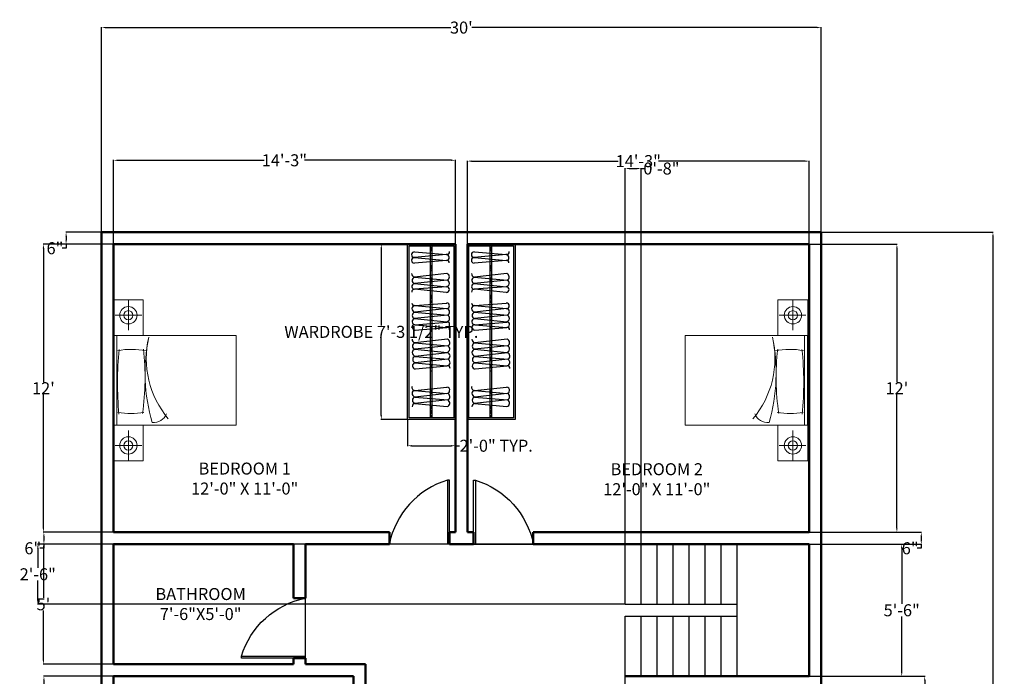
# Model space of a CAD drawing. Units: inches. Extents: x 20 to 32681, y 45 to 3082.
# Tile 3 of 5: x 20 to 512, y 344 to 672. Entities that reach past the tile are written whole.
import ezdxf

# ---------------------------------------------------------------- set-up
doc = ezdxf.new("R2010")
doc.units = ezdxf.units.IN
doc.header["$MEASUREMENT"] = 0
for name, color, linetype, lineweight in [('A-ANNO-DIMS', 2, 'Continuous', 18), ('A-AREA-IDEN', 7, 'Continuous', 25), ('A-DOOR', 4, 'Continuous', 25), ('A-FLOR-CASE', 32, 'Continuous', 25), ('A-FLOR-STRS', 3, 'Continuous', 25), ('A-FURN', 8, 'Continuous', 18), ('A-WALL', 7, 'Continuous', 50)]:
    doc.layers.add(name, color=color, linetype=linetype, lineweight=lineweight)
doc.styles.get("Standard").update_dxf_attribs({"font": 'arial.ttf'})
doc.dimstyles.get("Standard").update_dxf_attribs({"dimtxt": 6, "dimasz": 2, "dimexe": 0.18, "dimexo": 0.0625, "dimgap": 0.09, "dimtad": 0, "dimtih": 1, "dimtoh": 1, "dimdec": 0, "dimzin": 0, "dimdsep": 46, "dimlunit": 4, "dimtxsty": 'Standard', "dimcen": 0.09, "dimadec": 0, "dimazin": 0, "dimtfac": 1, "dimtdec": 0, "dimtofl": 0, "dimtmove": 0, "dimatfit": 3, "dimfxl": 1, "dimtolj": 1, "dimtzin": 0, "dimarcsym": 0})

# ---------------------------------------------------------------- blocks, each defined once
blk = doc.blocks.new('*D1')
at = {"layer": 'A-ANNO-DIMS', "color": 0, "lineweight": -2, "transparency": 16777216}
for p, q in [((60.79, 565.64), (60.79, 668.07)), ((62.79, 667.89), (235.61, 667.89)), ((418.79, 667.89), (245.97, 667.89)), ((420.79, 565.64), (420.79, 668.07))]:
    blk.add_line(p, q, dxfattribs=at)
at = {"layer": 'A-ANNO-DIMS', "color": 0, "transparency": 16777216}
for points in [[(62.79, 668.22), (62.79, 667.56), (60.79, 667.89)], [(418.79, 668.22), (418.79, 667.56), (420.79, 667.89)]]:
    blk.add_solid(points, dxfattribs=at)
at = {"layer": 'Defpoints', "color": 0, "transparency": 16777216}
for p in [(420.79, 667.89), (60.79, 565.58), (420.79, 565.58)]:
    blk.add_point(p, dxfattribs=at)
at = {"layer": 'A-ANNO-DIMS', "color": 0, "transparency": 16777216, "insert": (240.79, 667.89), "char_height": 6, "attachment_point": 5}
blk.add_mtext("\\A1;30'", dxfattribs=at)
blk = doc.blocks.new('DOOR')
for p, q in [((234.79, 441.58), (233.79, 441.58)), ((233.79, 441.58), (233.79, 409.58)), ((234.79, 409.58), (234.79, 441.58)), ((234.79, 409.58), (204.79, 409.58))]:
    blk.add_line(p, q)
blk.add_arc((245.82, 401.53), 41.82, 106.7253, 168.9058)
blk = doc.blocks.new('*D3')
at = {"layer": 'A-ANNO-DIMS', "color": 0, "lineweight": -2, "transparency": 16777216}
for p, q in [((414.85, 409.58), (461.22, 409.58)), ((461.04, 407.58), (461.04, 379.73)), ((461.04, 345.58), (461.04, 373.42)), ((414.85, 343.58), (461.22, 343.58))]:
    blk.add_line(p, q, dxfattribs=at)
at = {"layer": 'A-ANNO-DIMS', "color": 0, "transparency": 16777216}
for points in [[(460.7, 407.58), (461.37, 407.58), (461.04, 409.58)], [(460.7, 345.58), (461.37, 345.58), (461.04, 343.58)]]:
    blk.add_solid(points, dxfattribs=at)
at = {"layer": 'Defpoints', "color": 0, "transparency": 16777216}
for p in [(414.79, 409.58), (461.04, 409.58), (414.79, 343.58)]:
    blk.add_point(p, dxfattribs=at)
at = {"layer": 'A-ANNO-DIMS', "color": 0, "transparency": 16777216, "insert": (461.04, 376.58), "char_height": 6, "attachment_point": 5}
blk.add_mtext('\\A1;5\'-6"', dxfattribs=at)
blk = doc.blocks.new('CVBN')
for p, q in [((70.94, 1179.16), (70.94, 1191.01)), ((89.36, 1192.66), (89.36, 1168.36)), ((89.36, 1081.69), (89.36, 1192.39)), ((89.36, 1192.39), (89.36, 1168.09)), ((170.36, 1192.39), (89.36, 1192.39)), ((170.36, 1189.69), (89.36, 1189.69)), ((170.36, 1192.66), (170.36, 1168.36)), ((170.36, 1081.69), (170.36, 1192.39)), ((170.36, 1192.39), (170.36, 1168.09)), ((170.36, 1192.39), (170.36, 1168.09)), ((188.79, 1179.16), (188.79, 1191.01)), ((70.94, 1179.16), (56.8, 1179.16)), ((70.94, 1179.16), (84.43, 1179.16)), ((70.94, 1179.16), (70.94, 1166.85)), ((188.79, 1179.16), (175.29, 1179.16)), ((188.79, 1179.16), (202.93, 1179.16)), ((188.79, 1179.16), (188.79, 1166.85)), ((170.36, 1081.69), (89.36, 1081.69))]:
    blk.add_line(p, q)
for points in [[(56.96, 1192.66), (56.96, 1165.66), (89.36, 1165.66), (89.36, 1192.66)], [(202.76, 1192.66), (202.76, 1165.66), (170.36, 1165.66), (170.36, 1192.66)]]:
    blk.add_lwpolyline(points, close=True)
for centre, radius in [((70.94, 1179.16), 7.85), ((188.79, 1179.16), 7.85), ((70.94, 1179.16), 4.15), ((188.79, 1179.16), 4.15)]:
    blk.add_circle(centre, radius)
for centre, radius, start, end in [((127.34, 900.05), 288.94, 83.95302, 95.56263), ((165.23, 1177.16), 65.44, 169.91453, 190.68509), ((88.06, 1176.29), 69.84, 349.17608, 10.27064), ((136.55, 1004.48), 159.53, 78.24617, 106.34733), ((149.51, 1078.87), 84.09, 76.5636, 130.32358), ((132.8, 1394.24), 230.23, 261.76494, 276.28962), ((104.49, 1156.51), 12.88, 175.32687, 247.55878)]:
    blk.add_arc(centre, radius, start, end)
blk = doc.blocks.new('A$C1DC223CE')
for p, q in [((0, 600, -1029), (2200, 600, -1029)), ((0, 0, -1029), (0, 600, -1029)), ((20, 580, -1029), (2180, 580, -1029)), ((20, 20, -1029), (20, 580, -1029)), ((369, 495, -1029), (414, 88, -1029)), ((414, 85, -1029), (450, 501, -1029)), ((450, 499, -1029), (494, 87, -1029)), ((809, 498, -1029), (855, 91, -1029)), ((855, 88, -1029), (890, 504, -1029)), ((890, 502, -1029), (934, 89, -1029)), ((1194, 500, -1029), (1239, 93, -1029)), ((1239, 90, -1029), (1275, 506, -1029)), ((1275, 505, -1029), (1319, 92, -1029)), ((1319, 90, -1029), (1358, 496, -1029)), ((1363, 503, -1029), (1408, 96, -1029)), ((1408, 93, -1029), (1444, 509, -1029)), ((1444, 507, -1029), (1488, 95, -1029)), ((1488, 93, -1029), (1527, 499, -1029)), ((1565, 99, -1029), (1527, 499, -1029)), ((1874, 500, -1029), (1919, 93, -1029)), ((1919, 90, -1029), (1955, 506, -1029)), ((1955, 505, -1029), (1999, 92, -1029)), ((1999, 90, -1029), (2037, 496, -1029)), ((2180, 580, -1029), (2180, 20, -1029)), ((2200, 600, -1029), (2200, 0, -1029)), ((95, 88, -1029), (128, 488, -1029)), ((128, 486, -1029), (166, 85, -1029)), ((165, 88, -1029), (204, 488, -1029)), ((204, 488, -1029), (237, 85, -1029)), ((494, 85, -1029), (533, 491, -1029)), ((533, 488, -1029), (566, 85, -1029)), ((604, 488, -1029), (566, 88, -1029)), ((771, 91, -1029), (738, 491, -1029)), ((771, 91, -1029), (809, 491, -1029)), ((934, 88, -1029), (973, 494, -1029)), ((1011, 93, -1029), (979, 494, -1029)), ((1011, 93, -1029), (1045, 494, -1029)), ((1078, 93, -1029), (1045, 494, -1029)), ((1835, 92, -1029), (1795, 493, -1029)), ((1835, 93, -1029), (1874, 494, -1029)), ((2180, 309, -1029), (20, 309, -1029)), ((2180, 288, -1029), (20, 288, -1029)), ((45, 309, -1029), (45, 288, -1029)), ((50, 309, -1029), (50, 288, -1029)), ((63, 309, -1029), (63, 288, -1029)), ((77, 309, -1029), (77, 288, -1029)), ((83, 309, -1029), (83, 288, -1029)), ((273, 309, -1029), (273, 288, -1029)), ((278, 309, -1029), (278, 288, -1029)), ((291, 309, -1029), (291, 288, -1029)), ((304, 309, -1029), (304, 288, -1029)), ((313, 309, -1029), (313, 288, -1029)), ((333, 309, -1029), (333, 288, -1029)), ((428, 309, -1029), (428, 288, -1029)), ((433, 309, -1029), (433, 288, -1029)), ((446, 309, -1029), (446, 288, -1029)), ((459, 309, -1029), (459, 288, -1029)), ((468, 309, -1029), (468, 288, -1029)), ((488, 309, -1029), (488, 288, -1029)), ((645, 309, -1029), (645, 288, -1029)), ((650, 309, -1029), (650, 288, -1029)), ((660, 309, -1029), (660, 288, -1029)), ((678, 309, -1029), (678, 288, -1029)), ((683, 309, -1029), (683, 288, -1029)), ((687, 309, -1029), (687, 288, -1029)), ((716, 309, -1029), (716, 288, -1029)), ((725, 309, -1029), (725, 288, -1029)), ((731, 309, -1029), (731, 288, -1029)), ((877, 309, -1029), (877, 288, -1029)), ((888, 309, -1029), (888, 288, -1029)), ((952, 309, -1029), (952, 288, -1029)), ((959, 309, -1029), (959, 288, -1029)), ((1036, 309, -1029), (1036, 288, -1029)), ((1047, 309, -1029), (1047, 288, -1029)), ((1273, 309, -1029), (1273, 288, -1029)), ((1308, 309, -1029), (1308, 288, -1029)), ((1319, 309, -1029), (1319, 288, -1029)), ((1330, 309, -1029), (1330, 288, -1029)), ((1341, 309, -1029), (1341, 288, -1029)), ((1346, 309, -1029), (1346, 288, -1029)), ((1421, 309, -1029), (1421, 288, -1029)), ((1432, 309, -1029), (1432, 288, -1029)), ((1446, 309, -1029), (1446, 288, -1029)), ((1448, 309, -1029), (1448, 288, -1029)), ((1459, 309, -1029), (1459, 288, -1029)), ((1466, 309, -1029), (1466, 288, -1029)), ((1513, 309, -1029), (1513, 288, -1029)), ((1521, 309, -1029), (1521, 288, -1029)), ((1532, 309, -1029), (1532, 288, -1029)), ((1544, 309, -1029), (1544, 288, -1029)), ((1553, 309, -1029), (1553, 288, -1029)), ((1592, 309, -1029), (1592, 288, -1029)), ((1836, 309, -1029), (1836, 288, -1029)), ((1844, 309, -1029), (1844, 288, -1029)), ((1856, 309, -1029), (1856, 288, -1029)), ((1865, 309, -1029), (1865, 288, -1029)), ((1874, 309, -1029), (1874, 288, -1029)), ((2043, 309, -1029), (2043, 288, -1029)), ((2048, 309, -1029), (2048, 288, -1029)), ((2066, 309, -1029), (2066, 288, -1029)), ((2091, 309, -1029), (2091, 288, -1029)), ((2099, 309, -1029), (2099, 288, -1029)), ((2109, 309, -1029), (2109, 288, -1029)), ((2127, 309, -1029), (2127, 288, -1029)), ((2153, 309, -1029), (2153, 288, -1029)), ((2164, 309, -1029), (2164, 288, -1029)), ((2200, 0, -1029), (0, 0, -1029)), ((2180, 20, -1029), (20, 20, -1029))]:
    blk.add_line(p, q)
for centre, radius, start, end in [((98, 496, -1029), 31, 344.0746, 99.05), ((166, 484, -1029), 38.5, 94.0153, 178.1465), ((171, 491, -1029), 32.8, 355.4947, 103.6477), ((232, 494, -1029), 29, 86.5574, 190.9577), ((411, 482, -1029), 43.6, 25.0318, 162.7252), ((490, 482, -1029), 43.5, 11.8045, 156.7744), ((571, 487, -1029), 38.5, 94.0153, 178.1465), ((566, 487, -1029), 38.5, 1.8535, 85.9847), ((769, 494, -1029), 31.7, 82.3676, 185.3857), ((778, 494, -1029), 31.7, 354.6143, 97.6324), ((851, 485, -1029), 43.6, 25.0318, 162.7252), ((930, 485, -1029), 43.5, 11.8045, 156.7744), ((1002, 504, -1029), 25.4, 75.2713, 202.7917), ((1013, 497, -1029), 31.7, 354.6143, 97.6324), ((1068, 504, -1029), 25.4, 75.2713, 202.7917), ((1235, 488, -1029), 43.6, 25.0318, 162.7252), ((1315, 487, -1029), 43.5, 11.8045, 156.7744), ((1405, 490, -1029), 43.6, 25.0318, 162.7252), ((1484, 490, -1029), 43.5, 11.8045, 156.7744), ((1558, 502, -1029), 31.7, 82.3676, 185.3857), ((1830, 494, -1029), 35.9, 71.1886, 180.696), ((1842, 497, -1029), 31.7, 354.6143, 97.6324), ((1915, 488, -1029), 43.6, 25.0318, 162.7252), ((1995, 487, -1029), 43.5, 11.8045, 156.7744), ((133, 89, -1029), 38.5, 181.8535, 265.9847), ((135, 82, -1029), 31.7, 262.3676, 5.3857), ((204, 89, -1029), 38.5, 181.8535, 265.9847), ((205, 82, -1029), 31.7, 262.3676, 5.3857), ((364, 104, -1029), 52.8, 272.4772, 342.818), ((454, 98, -1029), 41.7, 197.7504, 344.2252), ((536, 96, -1029), 42.8, 195.0477, 270), ((529, 90, -1029), 37.5, 280.6806, 351.7243), ((597, 85, -1029), 31.7, 174.6143, 277.6324), ((742, 84, -1029), 30.1, 267.7337, 14.6117), ((809, 92, -1029), 38.5, 181.8535, 265.9847), ((804, 106, -1029), 52.8, 272.4772, 342.818), ((894, 101, -1029), 41.7, 197.7504, 344.2252), ((976, 99, -1029), 42.8, 195.0477, 270), ((973, 95, -1029), 38.5, 274.0153, 358.1465), ((1040, 86, -1029), 29.8, 166.1294, 272.546), ((1039, 95, -1029), 38.5, 274.0153, 358.1465), ((1189, 109, -1029), 52.8, 272.4772, 342.818), ((1279, 103, -1029), 41.7, 197.7504, 344.2252), ((1360, 101, -1029), 42.8, 195.0477, 270), ((1358, 111, -1029), 52.8, 272.4772, 342.818), ((1448, 106, -1029), 41.7, 197.7504, 344.2252), ((1530, 104, -1029), 42.8, 195.0477, 270), ((1527, 100, -1029), 38.5, 274.0153, 358.1465), ((1799, 90, -1029), 36.2, 250.2345, 4.119), ((1874, 94, -1029), 38.5, 181.8535, 265.9847), ((1869, 109, -1029), 52.8, 272.4772, 342.818), ((1959, 103, -1029), 41.7, 197.7504, 344.2252), ((2040, 101, -1029), 42.8, 195.0477, 270)]:
    blk.add_arc(centre, radius, start, end)
blk = doc.blocks.new('*D12')
at = {"layer": 'A-ANNO-DIMS', "color": 0, "lineweight": -2, "transparency": 16777216}
for p, q in [((60.73, 565.58), (42.93, 565.58)), ((43.11, 563.58), (43.11, 561.58)), ((43.11, 557.58), (41.11, 557.58)), ((60.73, 559.58), (42.93, 559.58)), ((43.11, 559.58), (43.11, 557.58))]:
    blk.add_line(p, q, dxfattribs=at)
at = {"layer": 'A-ANNO-DIMS', "color": 0, "transparency": 16777216}
for points in [[(42.78, 563.58), (43.44, 563.58), (43.11, 565.58)], [(42.78, 561.58), (43.44, 561.58), (43.11, 559.58)]]:
    blk.add_solid(points, dxfattribs=at)
at = {"layer": 'Defpoints', "color": 0, "transparency": 16777216}
for p in [(60.79, 565.58), (43.11, 559.58), (60.79, 559.58)]:
    blk.add_point(p, dxfattribs=at)
at = {"layer": 'A-ANNO-DIMS', "color": 0, "transparency": 16777216, "insert": (37.55, 557.58), "char_height": 6, "attachment_point": 5}
blk.add_mtext('\\A1;6"', dxfattribs=at)
blk = doc.blocks.new('*D13')
at = {"layer": 'A-ANNO-DIMS', "color": 0, "lineweight": -2, "transparency": 16777216}
for p, q in [((66.73, 559.58), (31.59, 559.58)), ((31.77, 557.58), (31.77, 490.68)), ((31.77, 417.58), (31.77, 484.47)), ((66.73, 415.58), (31.59, 415.58))]:
    blk.add_line(p, q, dxfattribs=at)
at = {"layer": 'A-ANNO-DIMS', "color": 0, "transparency": 16777216}
for points in [[(31.43, 557.58), (32.1, 557.58), (31.77, 559.58)], [(31.43, 417.58), (32.1, 417.58), (31.77, 415.58)]]:
    blk.add_solid(points, dxfattribs=at)
at = {"layer": 'Defpoints', "color": 0, "transparency": 16777216}
for p in [(66.79, 559.58), (31.77, 415.58), (66.79, 415.58)]:
    blk.add_point(p, dxfattribs=at)
at = {"layer": 'A-ANNO-DIMS', "color": 0, "transparency": 16777216, "insert": (31.77, 487.58), "char_height": 6, "attachment_point": 5}
blk.add_mtext("\\A1;12'", dxfattribs=at)
blk = doc.blocks.new('*D14')
at = {"layer": 'A-ANNO-DIMS', "color": 0, "lineweight": -2, "transparency": 16777216}
for p, q in [((66.73, 415.58), (31.83, 415.58)), ((66.73, 409.58), (31.83, 409.58)), ((32.01, 413.58), (32.01, 411.58)), ((32.01, 409.58), (32.01, 407.58)), ((32.01, 407.58), (30.01, 407.58))]:
    blk.add_line(p, q, dxfattribs=at)
at = {"layer": 'A-ANNO-DIMS', "color": 0, "transparency": 16777216}
for points in [[(31.68, 413.58), (32.34, 413.58), (32.01, 415.58)], [(31.68, 411.58), (32.34, 411.58), (32.01, 409.58)]]:
    blk.add_solid(points, dxfattribs=at)
at = {"layer": 'Defpoints', "color": 0, "transparency": 16777216}
for p in [(66.79, 415.58), (32.01, 409.58), (66.79, 409.58)]:
    blk.add_point(p, dxfattribs=at)
at = {"layer": 'A-ANNO-DIMS', "color": 0, "transparency": 16777216, "insert": (26.46, 407.58), "char_height": 6, "attachment_point": 5}
blk.add_mtext('\\A1;6"', dxfattribs=at)
blk = doc.blocks.new('*D15')
at = {"layer": 'A-ANNO-DIMS', "color": 0, "lineweight": -2, "transparency": 16777216}
for p, q in [((66.73, 409.58), (31.59, 409.58)), ((31.77, 407.58), (31.77, 382.72)), ((31.77, 351.58), (31.77, 376.43)), ((66.73, 349.58), (31.59, 349.58))]:
    blk.add_line(p, q, dxfattribs=at)
at = {"layer": 'A-ANNO-DIMS', "color": 0, "transparency": 16777216}
for points in [[(31.43, 407.58), (32.1, 407.58), (31.77, 409.58)], [(31.43, 351.58), (32.1, 351.58), (31.77, 349.58)]]:
    blk.add_solid(points, dxfattribs=at)
at = {"layer": 'Defpoints', "color": 0, "transparency": 16777216}
for p in [(66.79, 409.58), (31.77, 349.58), (66.79, 349.58)]:
    blk.add_point(p, dxfattribs=at)
at = {"layer": 'A-ANNO-DIMS', "color": 0, "transparency": 16777216, "insert": (31.77, 379.58), "char_height": 6, "attachment_point": 5}
blk.add_mtext("\\A1;5'", dxfattribs=at)
blk = doc.blocks.new('*D16')
at = {"layer": 'A-ANNO-DIMS', "color": 0, "lineweight": -2, "transparency": 16777216}
for p, q in [((66.73, 343.58), (31.84, 343.58)), ((32.02, 341.58), (32.02, 298.73)), ((32.02, 249.58), (32.02, 292.42)), ((66.73, 247.58), (31.84, 247.58))]:
    blk.add_line(p, q, dxfattribs=at)
at = {"layer": 'A-ANNO-DIMS', "color": 0, "transparency": 16777216}
for points in [[(31.69, 341.58), (32.35, 341.58), (32.02, 343.58)], [(31.69, 249.58), (32.35, 249.58), (32.02, 247.58)]]:
    blk.add_solid(points, dxfattribs=at)
at = {"layer": 'Defpoints', "color": 0, "transparency": 16777216}
for p in [(66.79, 343.58), (32.02, 247.58), (66.79, 247.58)]:
    blk.add_point(p, dxfattribs=at)
at = {"layer": 'A-ANNO-DIMS', "color": 0, "transparency": 16777216, "insert": (32.02, 295.58), "char_height": 6, "attachment_point": 5}
blk.add_mtext("\\A1;8'", dxfattribs=at)
blk = doc.blocks.new('*D22')
at = {"layer": 'A-ANNO-DIMS', "color": 0, "lineweight": -2, "transparency": 16777216}
for p, q in [((414.85, 343.58), (472.74, 343.58)), ((472.56, 341.58), (472.56, 339.58)), ((414.85, 337.58), (472.74, 337.58)), ((472.56, 335.58), (470.56, 335.58)), ((472.56, 337.58), (472.56, 335.58))]:
    blk.add_line(p, q, dxfattribs=at)
at = {"layer": 'A-ANNO-DIMS', "color": 0, "transparency": 16777216}
for points in [[(472.23, 341.58), (472.89, 341.58), (472.56, 343.58)], [(472.23, 339.58), (472.89, 339.58), (472.56, 337.58)]]:
    blk.add_solid(points, dxfattribs=at)
at = {"layer": 'Defpoints', "color": 0, "transparency": 16777216}
for p in [(414.79, 343.58), (414.79, 337.58), (472.56, 337.58)]:
    blk.add_point(p, dxfattribs=at)
at = {"layer": 'A-ANNO-DIMS', "color": 0, "transparency": 16777216, "insert": (467, 335.58), "char_height": 6, "attachment_point": 5}
blk.add_mtext('\\A1;6"', dxfattribs=at)
blk = doc.blocks.new('*D23')
at = {"layer": 'A-ANNO-DIMS', "color": 0, "lineweight": -2, "transparency": 16777216}
for p, q in [((414.85, 559.58), (458.81, 559.58)), ((458.63, 557.58), (458.63, 490.68)), ((458.63, 417.58), (458.63, 484.47)), ((414.85, 415.58), (458.81, 415.58))]:
    blk.add_line(p, q, dxfattribs=at)
at = {"layer": 'A-ANNO-DIMS', "color": 0, "transparency": 16777216}
for points in [[(458.3, 557.58), (458.97, 557.58), (458.63, 559.58)], [(458.3, 417.58), (458.97, 417.58), (458.63, 415.58)]]:
    blk.add_solid(points, dxfattribs=at)
at = {"layer": 'Defpoints', "color": 0, "transparency": 16777216}
for p in [(414.79, 559.58), (458.63, 559.58), (414.79, 415.58)]:
    blk.add_point(p, dxfattribs=at)
at = {"layer": 'A-ANNO-DIMS', "color": 0, "transparency": 16777216, "insert": (458.63, 487.58), "char_height": 6, "attachment_point": 5}
blk.add_mtext("\\A1;12'", dxfattribs=at)
blk = doc.blocks.new('*D24')
at = {"layer": 'A-ANNO-DIMS', "color": 0, "lineweight": -2, "transparency": 16777216}
for p, q in [((414.85, 415.58), (471.01, 415.58)), ((414.85, 409.58), (471.01, 409.58)), ((470.83, 413.58), (470.83, 411.58)), ((470.83, 409.58), (470.83, 407.58)), ((470.83, 407.58), (468.83, 407.58))]:
    blk.add_line(p, q, dxfattribs=at)
at = {"layer": 'A-ANNO-DIMS', "color": 0, "transparency": 16777216}
for points in [[(470.49, 413.58), (471.16, 413.58), (470.83, 415.58)], [(470.49, 411.58), (471.16, 411.58), (470.83, 409.58)]]:
    blk.add_solid(points, dxfattribs=at)
at = {"layer": 'Defpoints', "color": 0, "transparency": 16777216}
for p in [(414.79, 415.58), (414.79, 409.58), (470.83, 409.58)]:
    blk.add_point(p, dxfattribs=at)
at = {"layer": 'A-ANNO-DIMS', "color": 0, "transparency": 16777216, "insert": (465.27, 407.58), "char_height": 6, "attachment_point": 5}
blk.add_mtext('\\A1;6"', dxfattribs=at)
blk = doc.blocks.new('*D25')
at = {"layer": 'A-ANNO-DIMS', "color": 0, "lineweight": -2, "transparency": 16777216}
for p, q in [((243.79, 559.64), (243.79, 601.31)), ((245.79, 601.13), (319.18, 601.13)), ((412.79, 601.13), (339.4, 601.13)), ((414.79, 559.64), (414.79, 601.31))]:
    blk.add_line(p, q, dxfattribs=at)
at = {"layer": 'A-ANNO-DIMS', "color": 0, "transparency": 16777216}
for points in [[(245.79, 601.46), (245.79, 600.8), (243.79, 601.13)], [(412.79, 601.46), (412.79, 600.8), (414.79, 601.13)]]:
    blk.add_solid(points, dxfattribs=at)
at = {"layer": 'Defpoints', "color": 0, "transparency": 16777216}
for p in [(414.79, 601.13), (243.79, 559.58), (414.79, 559.58)]:
    blk.add_point(p, dxfattribs=at)
at = {"layer": 'A-ANNO-DIMS', "color": 0, "transparency": 16777216, "insert": (329.29, 601.13), "char_height": 6, "attachment_point": 5}
blk.add_mtext('\\A1;14\'-3"', dxfattribs=at)
blk = doc.blocks.new('*D26')
at = {"layer": 'A-ANNO-DIMS', "color": 0, "lineweight": -2, "transparency": 16777216}
for p, q in [((66.79, 559.64), (66.79, 601.72)), ((68.79, 601.54), (142.18, 601.54)), ((235.79, 601.54), (162.4, 601.54)), ((237.79, 559.64), (237.79, 601.72))]:
    blk.add_line(p, q, dxfattribs=at)
at = {"layer": 'A-ANNO-DIMS', "color": 0, "transparency": 16777216}
for points in [[(68.79, 601.88), (68.79, 601.21), (66.79, 601.54)], [(235.79, 601.88), (235.79, 601.21), (237.79, 601.54)]]:
    blk.add_solid(points, dxfattribs=at)
at = {"layer": 'Defpoints', "color": 0, "transparency": 16777216}
for p in [(237.79, 601.54), (66.79, 559.58), (237.79, 559.58)]:
    blk.add_point(p, dxfattribs=at)
at = {"layer": 'A-ANNO-DIMS', "color": 0, "transparency": 16777216, "insert": (152.29, 601.54), "char_height": 6, "attachment_point": 5}
blk.add_mtext('\\A1;14\'-3"', dxfattribs=at)
blk = doc.blocks.new('*D28')
at = {"layer": 'A-ANNO-DIMS', "color": 0, "lineweight": -2, "transparency": 16777216}
for p, q in [((420.85, 565.58), (506.85, 565.58)), ((506.67, 563.58), (506.67, 328.73)), ((506.67, 87.58), (506.67, 322.42)), ((420.85, 85.58), (506.85, 85.58))]:
    blk.add_line(p, q, dxfattribs=at)
at = {"layer": 'A-ANNO-DIMS', "color": 0, "transparency": 16777216}
for points in [[(506.34, 563.58), (507.01, 563.58), (506.67, 565.58)], [(506.34, 87.58), (507.01, 87.58), (506.67, 85.58)]]:
    blk.add_solid(points, dxfattribs=at)
at = {"layer": 'Defpoints', "color": 0, "transparency": 16777216}
for p in [(420.79, 565.58), (506.67, 565.58), (420.79, 85.58)]:
    blk.add_point(p, dxfattribs=at)
at = {"layer": 'A-ANNO-DIMS', "color": 0, "transparency": 16777216, "insert": (506.67, 325.58), "char_height": 6, "attachment_point": 5}
blk.add_mtext("\\A1;40'", dxfattribs=at)
blk = doc.blocks.new('*D34')
at = {"layer": 'A-ANNO-DIMS', "color": 0, "lineweight": -2, "transparency": 16777216}
for p, q in [((213.84, 559.58), (200.58, 559.58)), ((200.76, 557.58), (200.76, 518.97)), ((200.76, 473.98), (200.76, 512.58)), ((213.84, 471.98), (200.58, 471.98))]:
    blk.add_line(p, q, dxfattribs=at)
at = {"layer": 'A-ANNO-DIMS', "color": 0, "transparency": 16777216}
for points in [[(200.43, 557.58), (201.09, 557.58), (200.76, 559.58)], [(200.43, 473.98), (201.09, 473.98), (200.76, 471.98)]]:
    blk.add_solid(points, dxfattribs=at)
at = {"layer": 'Defpoints', "color": 0, "transparency": 16777216}
for p in [(213.9, 559.58), (200.76, 471.98), (213.9, 471.98)]:
    blk.add_point(p, dxfattribs=at)
at = {"layer": 'A-ANNO-DIMS', "color": 0, "transparency": 16777216, "insert": (200.76, 515.78), "char_height": 6, "attachment_point": 5}
blk.add_mtext('\\A1;WARDROBE 7\'-3 1/2" TYP.', dxfattribs=at)
blk = doc.blocks.new('*D35')
at = {"layer": 'A-ANNO-DIMS', "color": 0, "lineweight": -2, "transparency": 16777216}
for p, q in [((213.9, 471.91), (213.9, 458.66)), ((237.79, 471.91), (237.79, 458.66)), ((215.9, 458.84), (235.79, 458.84)), ((237.79, 458.84), (239.79, 458.84))]:
    blk.add_line(p, q, dxfattribs=at)
at = {"layer": 'A-ANNO-DIMS', "color": 0, "transparency": 16777216}
for points in [[(215.9, 459.17), (215.9, 458.5), (213.9, 458.84)], [(235.79, 459.17), (235.79, 458.5), (237.79, 458.84)]]:
    blk.add_solid(points, dxfattribs=at)
at = {"layer": 'Defpoints', "color": 0, "transparency": 16777216}
for p in [(213.9, 471.98), (237.79, 471.98), (237.79, 458.84)]:
    blk.add_point(p, dxfattribs=at)
at = {"layer": 'A-ANNO-DIMS', "color": 0, "transparency": 16777216, "insert": (258.22, 458.84), "char_height": 6, "attachment_point": 5}
blk.add_mtext('\\A1;2\'-0" TYP.', dxfattribs=at)
blk = doc.blocks.new('*D46')
at = {"layer": 'A-ANNO-DIMS', "color": 0, "lineweight": -2, "transparency": 16777216}
for p, q in [((322.73, 409.58), (28.76, 409.58)), ((28.94, 407.58), (28.94, 397.73)), ((28.94, 381.58), (28.94, 391.42)), ((322.73, 379.58), (28.76, 379.58))]:
    blk.add_line(p, q, dxfattribs=at)
at = {"layer": 'A-ANNO-DIMS', "color": 0, "transparency": 16777216}
for points in [[(28.61, 407.58), (29.27, 407.58), (28.94, 409.58)], [(28.61, 381.58), (29.27, 381.58), (28.94, 379.58)]]:
    blk.add_solid(points, dxfattribs=at)
at = {"layer": 'Defpoints', "color": 0, "transparency": 16777216}
for p in [(322.79, 409.58), (28.94, 379.58), (322.79, 379.58)]:
    blk.add_point(p, dxfattribs=at)
at = {"layer": 'A-ANNO-DIMS', "color": 0, "transparency": 16777216, "insert": (28.94, 394.58), "char_height": 6, "attachment_point": 5}
blk.add_mtext('\\A1;2\'-6"', dxfattribs=at)
blk = doc.blocks.new('*D47')
at = {"layer": 'A-ANNO-DIMS', "color": 0, "lineweight": -2, "transparency": 16777216}
for p, q in [((322.79, 409.64), (322.79, 597.61)), ((324.79, 597.43), (328.79, 597.43)), ((330.79, 409.64), (330.79, 597.61)), ((330.79, 597.43), (332.79, 597.43))]:
    blk.add_line(p, q, dxfattribs=at)
at = {"layer": 'A-ANNO-DIMS', "color": 0, "transparency": 16777216}
for points in [[(324.79, 597.76), (324.79, 597.09), (322.79, 597.43)], [(328.79, 597.76), (328.79, 597.09), (330.79, 597.43)]]:
    blk.add_solid(points, dxfattribs=at)
at = {"layer": 'Defpoints', "color": 0, "transparency": 16777216}
for p in [(330.79, 597.43), (322.79, 409.58), (330.79, 409.58)]:
    blk.add_point(p, dxfattribs=at)
at = {"layer": 'A-ANNO-DIMS', "color": 0, "transparency": 16777216, "insert": (340.86, 597.43), "char_height": 6, "attachment_point": 5}
blk.add_mtext('\\A1;0\'-8"', dxfattribs=at)

msp = doc.modelspace()

# ---------------------------------------------------------------- linework, layer by layer
at = {"layer": 'A-FLOR-STRS'}
for p, q in [((322.79, 379.58), (322.79, 409.58)), ((330.79, 379.58), (330.79, 409.58)), ((338.79, 379.58), (338.79, 409.58)), ((346.79, 379.58), (346.79, 409.58)), ((354.79, 379.58), (354.79, 409.58)), ((362.79, 379.58), (362.79, 409.58)), ((370.79, 379.58), (370.79, 409.58)), ((378.79, 343.58), (378.79, 409.58)), ((322.79, 379.58), (378.79, 379.58)), ((322.79, 373.58), (378.79, 373.58)), ((322.79, 337.58), (322.79, 373.58)), ((330.79, 343.58), (330.79, 373.58)), ((338.79, 343.58), (338.79, 373.58)), ((346.79, 343.58), (346.79, 373.58)), ((354.79, 343.58), (354.79, 373.58)), ((362.79, 343.58), (362.79, 373.58)), ((370.79, 343.58), (370.79, 373.58))]:
    msp.add_line(p, q, dxfattribs=at)
at = {"layer": 'A-WALL'}
for p, q in [((60.79, 565.58), (420.79, 565.58)), ((60.79, 565.58), (60.79, 85.58)), ((420.79, 85.58), (420.79, 565.58)), ((66.79, 559.58), (66.79, 415.58)), ((66.79, 559.58), (237.79, 559.58)), ((237.79, 559.58), (237.79, 415.58)), ((243.79, 559.58), (243.79, 415.58)), ((243.79, 559.58), (414.79, 559.58)), ((414.79, 415.58), (414.79, 559.58)), ((66.79, 415.58), (204.79, 415.58)), ((204.79, 415.58), (204.79, 409.58)), ((234.79, 415.58), (234.79, 409.58)), ((234.79, 415.58), (237.79, 415.58)), ((243.79, 415.58), (246.79, 415.58)), ((246.79, 415.58), (246.79, 409.58)), ((276.79, 415.58), (276.79, 409.58)), ((276.79, 415.58), (414.79, 415.58)), ((66.79, 409.58), (156.79, 409.58)), ((66.79, 409.58), (66.79, 349.58)), ((156.79, 409.58), (156.79, 382.58)), ((162.79, 409.58), (162.79, 382.58)), ((162.79, 409.58), (204.79, 409.58)), ((234.79, 409.58), (246.79, 409.58)), ((276.79, 409.58), (414.79, 409.58)), ((414.79, 343.58), (414.79, 409.58)), ((156.79, 382.58), (162.79, 382.58)), ((156.79, 352.58), (162.79, 352.58)), ((156.79, 352.58), (156.79, 349.58)), ((162.79, 352.58), (162.79, 349.58)), ((66.79, 349.58), (156.79, 349.58)), ((162.79, 349.58), (192.79, 349.58)), ((192.79, 349.58), (192.79, 283.58)), ((66.79, 343.58), (186.79, 343.58)), ((66.79, 343.58), (66.79, 247.58)), ((186.79, 343.58), (186.79, 283.58)), ((322.79, 343.58), (414.79, 343.58))]:
    msp.add_line(p, q, dxfattribs=at)

# ---------------------------------------------------------------- block references
at = {"layer": 'A-DOOR'}
msp.add_blockref('DOOR', (0, 0), dxfattribs=at)
at = {"layer": 'A-DOOR', "xscale": -1}
msp.add_blockref('DOOR', (481.58, 0), dxfattribs=at)
at = {"layer": 'A-DOOR', "xscale": -1, "rotation": 89.99999999999991}
msp.add_blockref('DOOR', (572.37, 587.37), dxfattribs=at)
at = {"layer": 'A-FLOR-CASE', "xscale": 0.039818128500731, "yscale": 0.039818128500731, "zscale": 0.039818128500731, "rotation": 270}
for p in [(213.9, 559.58, 40.96), (243.79, 559.58, 40.96)]:
    msp.add_blockref('A$C1DC223CE', p, dxfattribs=at)
at = {"layer": 'A-FURN', "yscale": 0.55247276188645, "zscale": 0.55247276188645}
for p, xscale, rotation in [((725.7, 419.78), 0.55247276188645, 90), ((-244.85, 419.78), -0.55247276188645, 270)]:
    msp.add_blockref('CVBN', p, dxfattribs=dict(at, xscale=xscale, rotation=rotation))

# ---------------------------------------------------------------- texts
at = {"layer": 'A-AREA-IDEN', "char_height": 6, "attachment_point": 1}
for s, width, insert in [('\\pxqc;BEDROOM 1\\P12\'-0" X 11\'-0"', 119.244, (72.82, 450.43)), ('\\pxqc;BEDROOM 2\\P12\'-0" X 11\'-0"', 119.244, (278.92, 450.11)), ('\\pxqc;BATHROOM\\P7\'-6"X5\'-0"', 128.6762, (46.07, 387.7))]:
    msp.add_mtext_dynamic_manual_height_columns(s, width=width, gutter_width=30, heights=[0], dxfattribs=dict(at, insert=insert))

# ---------------------------------------------------------------- dimensions: what is measured, and where the dimension line sits
at = {"layer": 'A-ANNO-DIMS'}
for base, p1, p2, override, picture, middle in [((420.79, 667.89), (60.79, 565.58), (420.79, 565.58), {"dimclrd": 0, "dimclre": 0, "dimclrt": 0}, '*D1', (240.79, 667.89)), ((237.79, 601.54), (66.79, 559.58), (237.79, 559.58), {"dimclrd": 0, "dimclre": 0, "dimclrt": 0}, '*D26', (152.29, 601.54)), ((414.79, 601.13), (243.79, 559.58), (414.79, 559.58), {"dimclrd": 0, "dimclre": 0, "dimclrt": 0}, '*D25', (329.29, 601.13)), ((330.79, 597.43), (322.79, 409.58), (330.79, 409.58), {"dimdec": 1, "dimlfac": 1, "dimrnd": 0, "dimzin": 1, "dimdsep": 46, "dimlunit": 4, "dimfrac": 2}, '*D47', (340.86, 597.43))]:
    dim = msp.add_linear_dim(base=base, p1=p1, p2=p2, dimstyle='Standard', override=override, dxfattribs=at)
    dim.commit()
    dim.dimension.update_dxf_attribs({"geometry": picture, "text_midpoint": middle})
for base, p1, p2, override, picture, middle in [((43.11, 559.58), (60.79, 565.58), (60.79, 559.58), {"dimclrd": 0, "dimclre": 0, "dimclrt": 0}, '*D12', (37.55, 557.58)), ((506.67, 565.58), (420.79, 85.58), (420.79, 565.58), {"dimclrd": 0, "dimclre": 0, "dimclrt": 0}, '*D28', (506.67, 325.58)), ((31.77, 415.58), (66.79, 559.58), (66.79, 415.58), {"dimclrd": 0, "dimclre": 0, "dimclrt": 0}, '*D13', (31.77, 487.58)), ((458.63, 559.58), (414.79, 415.58), (414.79, 559.58), {"dimclrd": 0, "dimclre": 0, "dimclrt": 0}, '*D23', (458.63, 487.58)), ((470.83, 409.58), (414.79, 415.58), (414.79, 409.58), {"dimclrd": 0, "dimclre": 0, "dimclrt": 0}, '*D24', (465.27, 407.58)), ((28.94, 379.58), (322.79, 409.58), (322.79, 379.58), {"dimdec": 1, "dimlfac": 1, "dimrnd": 0, "dimzin": 1, "dimdsep": 46, "dimlunit": 4, "dimfrac": 2}, '*D46', (28.94, 394.58)), ((31.77, 349.58), (66.79, 409.58), (66.79, 349.58), {"dimclrd": 0, "dimclre": 0, "dimclrt": 0}, '*D15', (31.77, 379.58)), ((461.04, 409.58), (414.79, 343.58), (414.79, 409.58), {"dimclrd": 0, "dimclre": 0, "dimclrt": 0}, '*D3', (461.04, 376.58)), ((32.02, 247.58), (66.79, 343.58), (66.79, 247.58), {"dimclrd": 0, "dimclre": 0, "dimclrt": 0}, '*D16', (32.02, 295.58)), ((472.56, 337.58), (414.79, 343.58), (414.79, 337.58), {"dimclrd": 0, "dimclre": 0, "dimclrt": 0}, '*D22', (467, 335.58))]:
    dim = msp.add_linear_dim(base=base, p1=p1, p2=p2, angle=90, dimstyle='Standard', override=override, dxfattribs=at)
    dim.commit()
    dim.dimension.update_dxf_attribs({"geometry": picture, "text_midpoint": middle})
dim = msp.add_linear_dim(base=(200.76, 471.98), p1=(213.9, 559.58), p2=(213.9, 471.98), angle=270, text='WARDROBE <> TYP.', dimstyle='Standard', override={"dimdec": 1, "dimlfac": 1, "dimrnd": 0, "dimzin": 1, "dimdsep": 46, "dimlunit": 4, "dimfrac": 2}, dxfattribs=at)
dim.commit()
dim.dimension.update_dxf_attribs({"geometry": '*D34', "text_midpoint": (200.76, 515.78)})
dim = msp.add_linear_dim(base=(237.79, 458.84), p1=(213.9, 471.98), p2=(237.79, 471.98), text='<> TYP.', dimstyle='Standard', override={"dimdec": 1, "dimlfac": 1, "dimrnd": 0, "dimzin": 1, "dimdsep": 46, "dimlunit": 4, "dimfrac": 2}, dxfattribs=at)
dim.commit()
dim.dimension.update_dxf_attribs({"geometry": '*D35', "text_midpoint": (258.22, 458.84)})
dim = msp.add_aligned_dim(p1=(66.79, 415.58), p2=(66.79, 409.58), distance=-34.78, dimstyle='Standard', override={"dimclrd": 0, "dimclre": 0, "dimclrt": 0}, dxfattribs=at)
dim.commit()
dim.dimension.update_dxf_attribs({"geometry": '*D14', "text_midpoint": (26.46, 407.58)})

doc.saveas('drawing.dxf')
